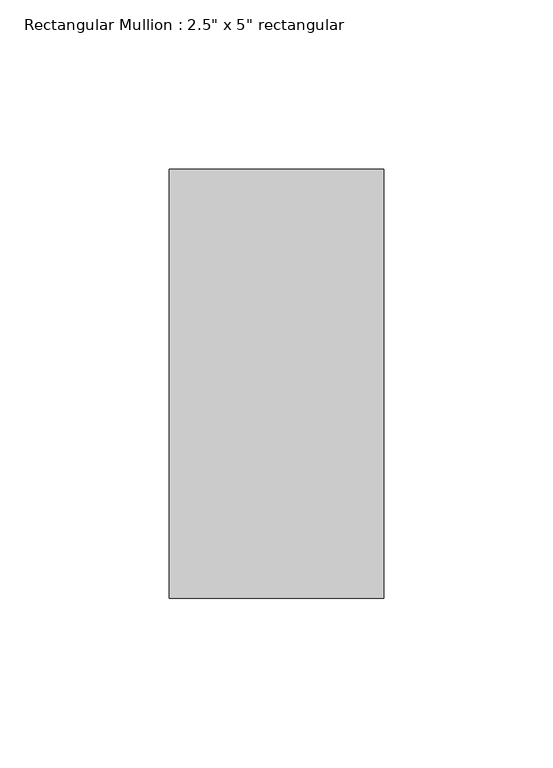
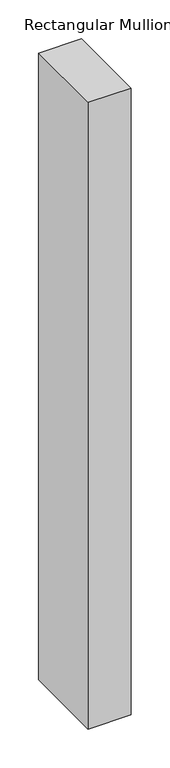
"""IFC4 building model written with IfcOpenShell, lengths in millimetres: member geometry."""

from ifc_helpers import new_model, si_unit, frame, origin, place, context, project, spatial, polyline, outline, extrude, source, transform, mapped, element, save


def member_eb4ec5b9(model_context):
    return source(origin(), model_context, "Body", "SweptSolid", [
        extrude(outline(polyline([(31.75, 63.5), (31.75, -63.5), (-31.75, -63.5), (-31.75, 63.5), (31.75, 63.5)])), frame((0.0, 0.0, -983.0744987), z_axis=(0.0, 0.0, 1.0), x_axis=(1.0, 0.0, 0.0)), (0.0, 0.0, 1.0), 983.0744987),
    ])


if __name__ == "__main__":
    model = new_model("IFC4")
    model_context = context("Model", 3, world=origin())
    ifc_project = project(units=[si_unit("LENGTHUNIT", "METRE", prefix="MILLI")], contexts=[model_context])
    site = spatial("IfcSite", under=ifc_project)
    building = spatial("IfcBuilding", under=site)
    placement = place(None, origin())
    member_shape = member_eb4ec5b9(model_context)
    element("IfcMember", 1, ObjectType="Rectangular Mullion : 2.5\" x 5\" rectangular", at=placement, inside=building, context=model_context, shape_type="MappedRepresentation", body=[
        mapped(member_shape, transform((0.0, 0.0, 0.0), x_axis=(1.0, 0.0, 0.0), y_axis=(0.0, 1.0, 0.0), z_axis=(0.0, 0.0, 1.0))),
    ])
    save(model, "model.ifc")

# Revit data of these elements
# Type "Rectangular Mullion : 2.5\" x 5\" rectangular"
#   built-in parameter 1007304 = 0.416667 (stored number, unit not read)
#   built-in parameter 1007301 = 0.104167 (stored number, unit not read)
#   built-in parameter 1007300 = 0.104167 (stored number, unit not read)
# Element 1 (IfcMember, "Rectangular Mullion : 2.5\" x 5\" rectangular")
#   Materials on its faces: "Aluminum"
# Materials
#   "Aluminum": class "Metal", colour RGB 247 247 247, transparency 0, Description = "Aluminum 6061", Cost = 0
